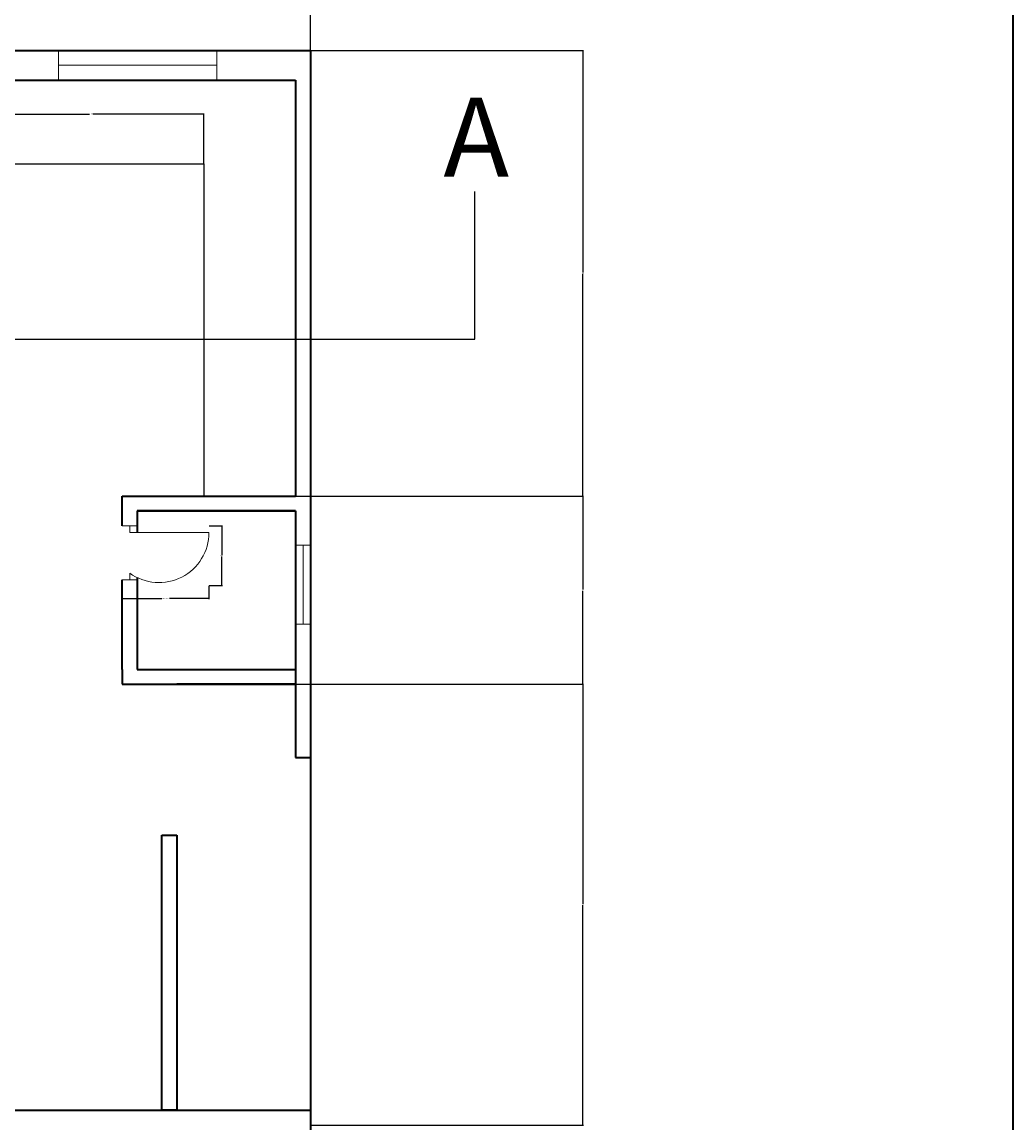
# Model space of a CAD drawing. Units: inches. Extents: x 2043 to 3387, y 1535 to 2797.
# Tile 6 of 7: x 3087 to 3387, y 2002 to 2335. Entities that reach past the tile are written whole.
import ezdxf

# ---------------------------------------------------------------- set-up
doc = ezdxf.new("R2010")
doc.units = ezdxf.units.IN
for name, color, linetype, lineweight in [('A-ANNO-DIMS', 2, 'Continuous', 18), ('A-ANNO-SYMB', 2, 'Continuous', 25), ('A-ANNO-TTLB', 7, 'Continuous', 35), ('A-DOOR', 3, 'Continuous', 18), ('A-FLOR-FIXT', 9, 'Continuous', 25), ('A-GLAZ', 4, 'Continuous', 18), ('A-WALL', 7, 'Continuous', 35)]:
    doc.layers.add(name, color=color, linetype=linetype, lineweight=lineweight)
doc.styles.get("Standard").update_dxf_attribs({"font": 'arial.ttf'})
doc.dimstyles.get("Standard").update_dxf_attribs({"dimtxt": 0.18, "dimasz": 0.18, "dimexe": 0.18, "dimexo": 0.0625, "dimgap": 0.09, "dimtad": 0, "dimtih": 1, "dimtoh": 1, "dimdec": 4, "dimzin": 0, "dimdsep": 46, "dimtxsty": 'Standard', "dimcen": 0.09, "dimadec": 0, "dimazin": 0, "dimtfac": 1, "dimtdec": 4, "dimtofl": 0, "dimtmove": 0, "dimatfit": 3, "dimfxl": 1, "dimtolj": 1, "dimtzin": 0, "dimarcsym": 0})

# ---------------------------------------------------------------- blocks, each defined once
blk = doc.blocks.new('DOOR-24-WC-NE')
for p, q in [((0, 17.14), (4.5, 17.14)), ((4.5, 17.14), (2.25, 17.14)), ((2.25, 17.14), (2.25, 15.14)), ((2.25, 15.14), (26.25, 15.14)), ((0, 0.86), (4.5, 0.86)), ((2.25, 0.86), (2.25, 2.86)), ((4.5, 0.86), (2.25, 0.86)), ((4.5, 0.86), (4.5, 0.86))]:
    blk.add_line(p, q)
blk.add_arc((11.11, 15.14), 15.14, 234.1954, 0)
blk = doc.blocks.new('COUNTER-L-NE')
for p, q in [((0, 100.61), (68.19, 100.61)), ((68.19, 100.61), (68.19, 0))]:
    blk.add_line(p, q)
blk = doc.blocks.new('WIN-48-PLAN')
for p, q in [((0, 9), (0, 0)), ((48, 4.5), (48, 9)), ((48, 9), (48, 0)), ((0, 0), (0, 4.5)), ((0, 4.5), (48, 4.5))]:
    blk.add_line(p, q)
blk = doc.blocks.new('VENT-24-PLAN')
for p, q in [((0, 24), (4.5, 24)), ((4.5, 24), (2.25, 24)), ((2.25, 24), (2.25, 0)), ((2.25, 0), (0, 0)), ((0, 0), (4.5, 0))]:
    blk.add_line(p, q)
blk = doc.blocks.new('*D51')
at = {"layer": 'A-ANNO-DIMS', "color": 0, "lineweight": -2, "transparency": 16777216}
for p, q in [((3117.21, 2164.2), (3117.21, 2160.15)), ((3143.46, 2164.2), (3143.46, 2160.15)), ((3117.39, 2160.33), (3129.15, 2160.33)), ((3143.28, 2160.33), (3131.52, 2160.33))]:
    blk.add_line(p, q, dxfattribs=at)
at = {"layer": 'A-ANNO-DIMS', "color": 0, "transparency": 16777216}
for points in [[(3117.39, 2160.36), (3117.39, 2160.3), (3117.21, 2160.33)], [(3143.28, 2160.36), (3143.28, 2160.3), (3143.46, 2160.33)]]:
    blk.add_solid(points, dxfattribs=at)
at = {"layer": 'Defpoints', "color": 0, "transparency": 16777216}
for p in [(3117.21, 2164.26), (3143.46, 2164.26), (3143.46, 2160.33)]:
    blk.add_point(p, dxfattribs=at)
at = {"layer": 'A-ANNO-DIMS', "color": 0, "transparency": 16777216, "insert": (3130.33, 2160.33), "char_height": 0.18, "attachment_point": 5}
blk.add_mtext('\\A1;WC DOOR 26 TYP.', dxfattribs=at)
blk = doc.blocks.new('*D52')
at = {"layer": 'A-ANNO-DIMS', "color": 0, "lineweight": -2, "transparency": 16777216}
for p, q in [((3143.52, 2182.33), (3147.58, 2182.33)), ((3147.4, 2182.15), (3147.4, 2173.48)), ((3147.4, 2164.44), (3147.4, 2173.12)), ((3143.52, 2164.26), (3147.58, 2164.26))]:
    blk.add_line(p, q, dxfattribs=at)
at = {"layer": 'A-ANNO-DIMS', "color": 0, "transparency": 16777216}
for points in [[(3147.37, 2182.15), (3147.43, 2182.15), (3147.4, 2182.33)], [(3147.37, 2164.44), (3147.43, 2164.44), (3147.4, 2164.26)]]:
    blk.add_solid(points, dxfattribs=at)
at = {"layer": 'Defpoints', "color": 0, "transparency": 16777216}
for p in [(3143.46, 2182.33), (3147.4, 2182.33), (3143.46, 2164.26)]:
    blk.add_point(p, dxfattribs=at)
at = {"layer": 'A-ANNO-DIMS', "color": 0, "transparency": 16777216, "insert": (3147.4, 2173.3), "char_height": 0.18, "attachment_point": 5}
blk.add_mtext('\\A1;18 TYP.', dxfattribs=at)
blk = doc.blocks.new('*D84')
at = {"layer": 'A-ANNO-DIMS', "color": 0, "lineweight": -2, "transparency": 16777216}
for p, q in [((3073.71, 2292.05), (3073.71, 2307.26)), ((3073.89, 2307.08), (3107.27, 2307.08)), ((3141.72, 2307.08), (3108.33, 2307.08)), ((3141.9, 2292.05), (3141.9, 2307.26))]:
    blk.add_line(p, q, dxfattribs=at)
at = {"layer": 'A-ANNO-DIMS', "color": 0, "transparency": 16777216}
for points in [[(3073.89, 2307.11), (3073.89, 2307.05), (3073.71, 2307.08)], [(3141.72, 2307.11), (3141.72, 2307.05), (3141.9, 2307.08)]]:
    blk.add_solid(points, dxfattribs=at)
at = {"layer": 'Defpoints', "color": 0, "transparency": 16777216}
for p in [(3141.9, 2307.08), (3073.71, 2291.99), (3141.9, 2291.99)]:
    blk.add_point(p, dxfattribs=at)
at = {"layer": 'A-ANNO-DIMS', "color": 0, "transparency": 16777216, "insert": (3107.8, 2307.08), "char_height": 0.18, "attachment_point": 5}
blk.add_mtext('\\A1;68 TYP.', dxfattribs=at)
blk = doc.blocks.new('*D110')
at = {"layer": 'A-ANNO-DIMS', "color": 0, "lineweight": -2, "transparency": 16777216}
for p, q in [((3069.21, 2317.44), (3069.21, 2359.26)), ((3069.39, 2359.08), (3121.43, 2359.08)), ((3174.03, 2359.08), (3121.99, 2359.08)), ((3174.21, 2326.44), (3174.21, 2359.26))]:
    blk.add_line(p, q, dxfattribs=at)
at = {"layer": 'A-ANNO-DIMS', "color": 0, "transparency": 16777216}
for points in [[(3069.39, 2359.11), (3069.39, 2359.05), (3069.21, 2359.08)], [(3174.03, 2359.11), (3174.03, 2359.05), (3174.21, 2359.08)]]:
    blk.add_solid(points, dxfattribs=at)
at = {"layer": 'Defpoints', "color": 0, "transparency": 16777216}
for p in [(3174.21, 2359.08), (3174.21, 2326.38), (3069.21, 2317.38)]:
    blk.add_point(p, dxfattribs=at)
at = {"layer": 'A-ANNO-DIMS', "color": 0, "transparency": 16777216, "insert": (3121.71, 2359.08), "char_height": 0.18, "attachment_point": 5}
blk.add_mtext('\\A1;105', dxfattribs=at)
blk = doc.blocks.new('*D114')
at = {"layer": 'A-ANNO-DIMS', "color": 0, "lineweight": -2, "transparency": 16777216}
for p, q in [((3169.77, 2134.38), (3256.85, 2134.38)), ((3256.67, 2134.2), (3256.67, 2067.81)), ((3256.67, 2001.06), (3256.67, 2067.44)), ((3174.27, 2000.88), (3256.85, 2000.88))]:
    blk.add_line(p, q, dxfattribs=at)
at = {"layer": 'A-ANNO-DIMS', "color": 0, "transparency": 16777216}
for points in [[(3256.64, 2134.2), (3256.7, 2134.2), (3256.67, 2134.38)], [(3256.64, 2001.06), (3256.7, 2001.06), (3256.67, 2000.88)]]:
    blk.add_solid(points, dxfattribs=at)
at = {"layer": 'Defpoints', "color": 0, "transparency": 16777216}
for p in [(3169.71, 2134.38), (3256.67, 2134.38), (3174.21, 2000.88)]:
    blk.add_point(p, dxfattribs=at)
at = {"layer": 'A-ANNO-DIMS', "color": 0, "transparency": 16777216, "insert": (3256.67, 2067.63), "char_height": 0.18, "attachment_point": 5}
blk.add_mtext('\\A1;133.5', dxfattribs=at)
blk = doc.blocks.new('*D115')
at = {"layer": 'A-ANNO-DIMS', "color": 0, "lineweight": -2, "transparency": 16777216}
for p, q in [((3169.77, 2191.38), (3256.85, 2191.38)), ((3256.67, 2191.2), (3256.67, 2163.06)), ((3256.67, 2134.56), (3256.67, 2162.7)), ((3169.77, 2134.38), (3256.85, 2134.38))]:
    blk.add_line(p, q, dxfattribs=at)
at = {"layer": 'A-ANNO-DIMS', "color": 0, "transparency": 16777216}
for points in [[(3256.64, 2191.2), (3256.7, 2191.2), (3256.67, 2191.38)], [(3256.64, 2134.56), (3256.7, 2134.56), (3256.67, 2134.38)]]:
    blk.add_solid(points, dxfattribs=at)
at = {"layer": 'Defpoints', "color": 0, "transparency": 16777216}
for p in [(3169.71, 2191.38), (3256.67, 2191.38), (3169.71, 2134.38)]:
    blk.add_point(p, dxfattribs=at)
at = {"layer": 'A-ANNO-DIMS', "color": 0, "transparency": 16777216, "insert": (3256.67, 2162.88), "char_height": 0.18, "attachment_point": 5}
blk.add_mtext('\\A1;57', dxfattribs=at)
blk = doc.blocks.new('*D116')
at = {"layer": 'A-ANNO-DIMS', "color": 0, "lineweight": -2, "transparency": 16777216}
for p, q in [((3174.27, 2326.38), (3256.85, 2326.38)), ((3256.67, 2326.2), (3256.67, 2259.06)), ((3256.67, 2191.56), (3256.67, 2258.69)), ((3169.77, 2191.38), (3256.85, 2191.38))]:
    blk.add_line(p, q, dxfattribs=at)
at = {"layer": 'A-ANNO-DIMS', "color": 0, "transparency": 16777216}
for points in [[(3256.64, 2326.2), (3256.7, 2326.2), (3256.67, 2326.38)], [(3256.64, 2191.56), (3256.7, 2191.56), (3256.67, 2191.38)]]:
    blk.add_solid(points, dxfattribs=at)
at = {"layer": 'Defpoints', "color": 0, "transparency": 16777216}
for p in [(3174.21, 2326.38), (3256.67, 2326.38), (3169.71, 2191.38)]:
    blk.add_point(p, dxfattribs=at)
at = {"layer": 'A-ANNO-DIMS', "color": 0, "transparency": 16777216, "insert": (3256.67, 2258.88), "char_height": 0.18, "attachment_point": 5}
blk.add_mtext('\\A1;135', dxfattribs=at)

msp = doc.modelspace()

# ---------------------------------------------------------------- linework, layer by layer
at = {"layer": 'A-ANNO-SYMB'}
for p, q in [((3223.9712, 2238.9239), (3223.9712, 2283.6261)), ((2693.0063, 2238.9239), (3223.9712, 2238.9239))]:
    msp.add_line(p, q, dxfattribs=at)
at = {"layer": 'A-ANNO-TTLB'}
msp.add_lwpolyline([(2042.5541, 2796.7818), (3386.9704, 2796.7818), (3386.9704, 1534.5689), (2042.5541, 1534.5689)], close=True, dxfattribs=at)
at = {"layer": 'A-WALL'}
for p, q in [((2723.7086, 2326.3769), (3174.2086, 2326.3769)), ((3174.2086, 2326.3769), (3174.2086, 1685.8769)), ((3073.7086, 2317.3769), (3169.7086, 2317.3769)), ((3169.7086, 2317.3769), (3169.7086, 2191.3769)), ((3117.2086, 2191.3769), (3169.7086, 2191.3769)), ((3117.2086, 2182.3328), (3117.2086, 2191.3769)), ((3121.7086, 2186.8769), (3169.7086, 2186.8769)), ((3169.7086, 2186.8769), (3121.7086, 2186.8769)), ((3121.7086, 2186.8769), (3121.7086, 2180.3328)), ((3169.7086, 2186.8769), (3169.7086, 2112.2282)), ((3117.2086, 2138.8769), (3117.2086, 2166.0526)), ((3121.7086, 2166.7092), (3121.7086, 2138.8769)), ((3117.2086, 2138.8769), (3117.2086, 2134.3769)), ((3121.7086, 2138.8769), (3169.7086, 2138.8769)), ((3117.2086, 2134.3769), (3169.7086, 2134.3769)), ((3169.7086, 2134.3769), (3133.7086, 2134.3769)), ((3169.7086, 2112.2282), (3174.2086, 2112.2282)), ((3129.2086, 2005.3769), (3129.2086, 2088.7241)), ((3129.2086, 2088.7241), (3133.7086, 2088.7241)), ((3133.7086, 2088.7241), (3133.7086, 2005.3769)), ((3002.2086, 2005.3769), (3174.2086, 2005.3769)), ((3133.7086, 2005.3769), (3129.2086, 2005.3769))]:
    msp.add_line(p, q, dxfattribs=at)

# ---------------------------------------------------------------- block references
at = {"layer": 'A-DOOR'}
msp.add_blockref('DOOR-24-WC-NE', (3117.209, 2165.192), dxfattribs=at)
at = {"layer": 'A-FLOR-FIXT'}
msp.add_blockref('COUNTER-L-NE', (3073.709, 2191.377), dxfattribs=at)
at = {"layer": 'A-GLAZ'}
msp.add_blockref('WIN-48-PLAN', (3097.8621, 2317.377), dxfattribs=at)
at = {"layer": 'A-GLAZ', "rotation": 180}
msp.add_blockref('VENT-24-PLAN', (3174.2082, 2176.5458), dxfattribs=at)

# ---------------------------------------------------------------- texts
at = {"layer": 'A-ANNO-SYMB', "insert": (3214.4394, 2312.0861), "char_height": 24, "attachment_point": 1}
msp.add_mtext_dynamic_manual_height_columns('A', width=23.218084, gutter_width=12.5, heights=[0], dxfattribs=at)

# ---------------------------------------------------------------- dimensions: what is measured, and where the dimension line sits
at = {"layer": 'A-ANNO-DIMS'}
dim = msp.add_linear_dim(base=(3174.2086, 2359.0769), p1=(3069.2086, 2317.3769), p2=(3174.2086, 2326.3769), dimstyle='Standard', override={"dimdec": 0, "dimlfac": 1, "dimrnd": 0, "dimzin": 0, "dimdsep": 46, "dimlunit": 2}, dxfattribs=at)
dim.commit()
dim.dimension.update_dxf_attribs({"geometry": '*D110', "text_midpoint": (3121.7086, 2359.0769)})
for base, p1, p2, override, picture, middle in [((3256.6712, 2326.3769), (3169.7086, 2191.3769), (3174.2086, 2326.3769), {"dimdec": 0, "dimlfac": 1, "dimrnd": 0, "dimzin": 0, "dimdsep": 46, "dimlunit": 2}, '*D116', (3256.6712, 2258.8769)), ((3256.6712, 2191.3769), (3169.7086, 2134.3769), (3169.7086, 2191.3769), {"dimdec": 0, "dimlfac": 1, "dimrnd": 0, "dimzin": 0, "dimdsep": 46, "dimlunit": 2}, '*D115', (3256.6712, 2162.8769)), ((3256.6712, 2134.3769), (3174.2086, 2000.8769), (3169.7086, 2134.3769), {"dimdec": 1, "dimlfac": 1, "dimrnd": 0, "dimzin": 0, "dimdsep": 46, "dimlunit": 2}, '*D114', (3256.6712, 2067.6269))]:
    dim = msp.add_linear_dim(base=base, p1=p1, p2=p2, angle=90, dimstyle='Standard', override=override, dxfattribs=at)
    dim.commit()
    dim.dimension.update_dxf_attribs({"geometry": picture, "text_midpoint": middle})
for base, p1, p2, text, picture, middle in [((3141.8962, 2307.0803), (3073.7086, 2291.9886), (3141.8962, 2291.9886), '<> TYP.', '*D84', (3107.8024, 2307.0803)), ((3143.4586, 2160.3263), (3117.2086, 2164.2638), (3143.4586, 2164.2638), 'WC DOOR <> TYP.', '*D51', (3130.3336, 2160.3263))]:
    dim = msp.add_linear_dim(base=base, p1=p1, p2=p2, text=text, dimstyle='Standard', override={"dimdec": 0, "dimlfac": 1, "dimrnd": 0, "dimzin": 0, "dimdsep": 46, "dimlunit": 2}, dxfattribs=at)
    dim.commit()
    dim.dimension.update_dxf_attribs({"geometry": picture, "text_midpoint": middle})
dim = msp.add_linear_dim(base=(3147.3961, 2182.3328), p1=(3143.4586, 2164.2638), p2=(3143.4586, 2182.3328), angle=90, text='<> TYP.', dimstyle='Standard', override={"dimdec": 0, "dimlfac": 1, "dimrnd": 0, "dimzin": 0, "dimdsep": 46, "dimlunit": 2}, dxfattribs=at)
dim.commit()
dim.dimension.update_dxf_attribs({"geometry": '*D52', "text_midpoint": (3147.3961, 2173.2983)})

doc.saveas('drawing.dxf')
